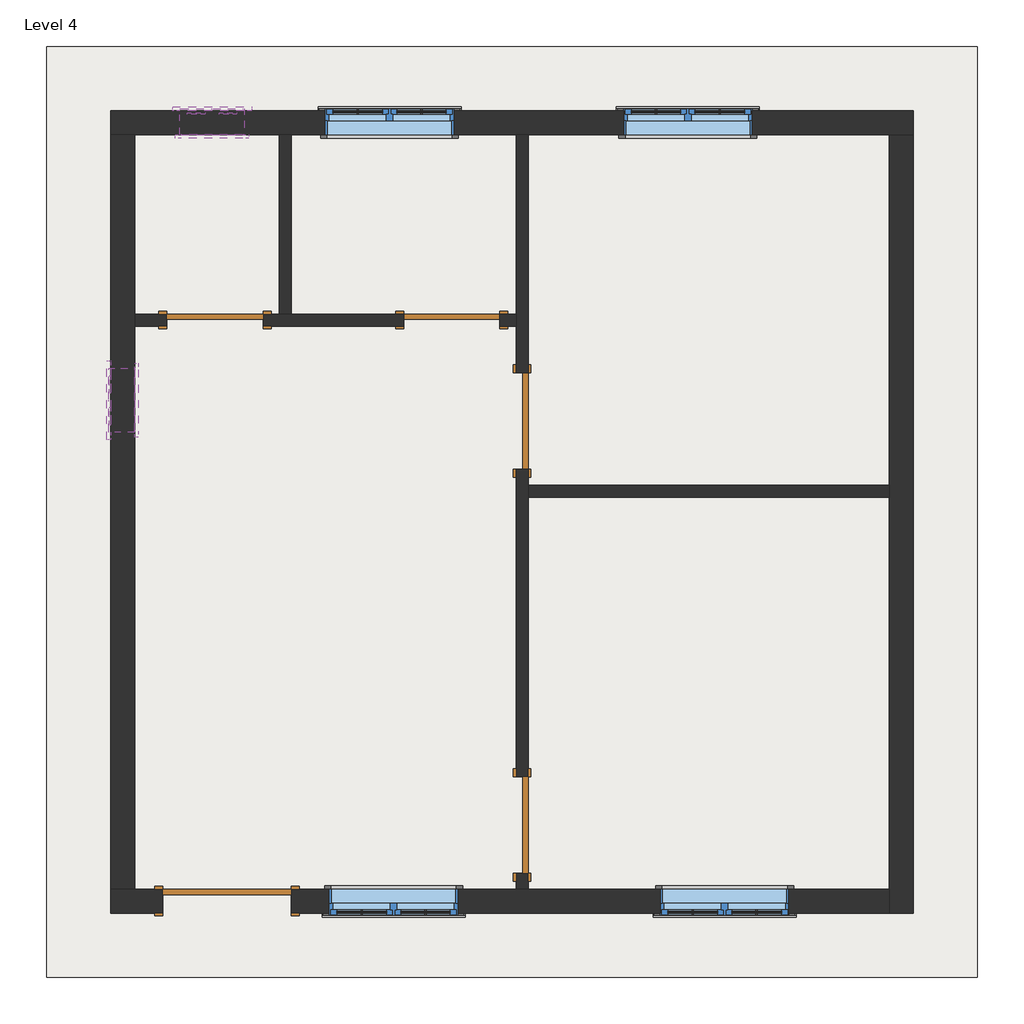
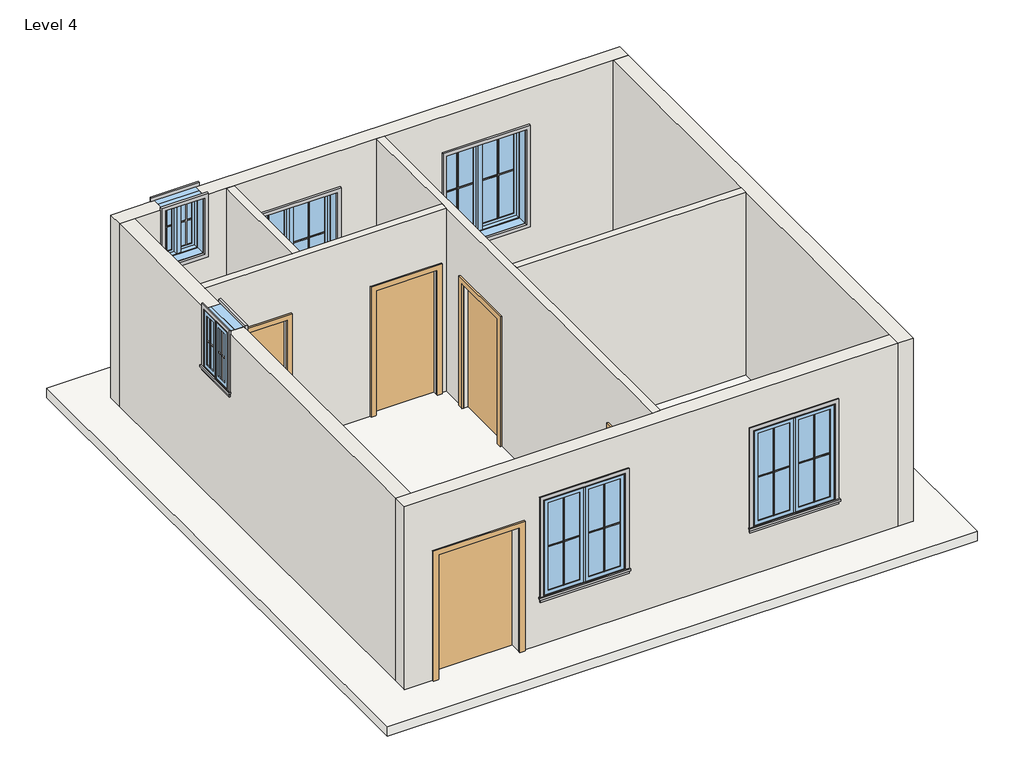
# One storey, incomplete: 24 proxies, 8 walls, 6 windows, 5 doors, 1 roof.
"""IFC4 building model written with IfcOpenShell, lengths in millimetres."""

from ifc_helpers import new_model, si_unit, frame, origin, place, context, project, spatial, polyline, outline, extrude, faceted_brep, transform, mapped, element, save
from components import muntin_pattern_2x2_muntin_pattern_2x2_6dad3731, muntin_pattern_2x2_muntin_pattern_2x2_a30a3345, muntin_pattern_2x2_muntin_pattern_2x2_53152e2c, muntin_pattern_2x2_muntin_pattern_2x2_e8f3e573, trim_window_exterior_flat_with_sill_92b9b949, trim_window_exterior_flat_with_sill_a665a915, trim_window_interior_flat_picture_frame_3bb882cf, trim_window_interior_flat_picture_frame_d485c387, door_e5f9f3c4, door_f4c4cdf2, window_c417fced, window_8377141f

model = new_model("IFC4")

# Units and contexts
model_context = context("Model", 3, world=origin())
ifc_project = project(units=[si_unit("LENGTHUNIT", "METRE", prefix="MILLI")], contexts=[model_context])

# Site, building, storey
site = spatial("IfcSite", under=ifc_project)
building = spatial("IfcBuilding", under=site)
storey = spatial("IfcBuildingStorey", under=building, Name="Level 4", Elevation=9144.0)

# Proxies
placement = place(None, origin())
muntin_pattern_2x2_muntin_pattern_2x2_shape = muntin_pattern_2x2_muntin_pattern_2x2_6dad3731(model_context)
element("IfcBuildingElementProxy", 1, Name="Muntin Pattern_2x2 : Muntin Pattern_2x2", ObjectType="Muntin Pattern_2x2 : Muntin Pattern_2x2", at=placement, inside=storey, context=model_context, shape_type="MappedRepresentation", body=[
    mapped(muntin_pattern_2x2_muntin_pattern_2x2_shape, transform((6192.8375, 13960.475, 10128.25), x_axis=(1.0, 0.0, 0.0), y_axis=(0.0, 1.0, 0.0), z_axis=(0.0, 0.0, 1.0))),
])
element("IfcBuildingElementProxy", 2, Name="Muntin Pattern_2x2 : Muntin Pattern_2x2", ObjectType="Muntin Pattern_2x2 : Muntin Pattern_2x2", at=placement, inside=storey, context=model_context, shape_type="MappedRepresentation", body=[
    mapped(muntin_pattern_2x2_muntin_pattern_2x2_shape, transform((7148.5125, 6359.525, 10128.25), x_axis=(-1.0, 0.0, 0.0), y_axis=(0.0, -1.0, 0.0), z_axis=(0.0, 0.0, 1.0))),
])
element("IfcBuildingElementProxy", 3, Name="Muntin Pattern_2x2 : Muntin Pattern_2x2", ObjectType="Muntin Pattern_2x2 : Muntin Pattern_2x2", at=placement, inside=storey, context=model_context, shape_type="MappedRepresentation", body=[
    mapped(muntin_pattern_2x2_muntin_pattern_2x2_shape, transform((4005.2625, 6359.525, 10128.25), x_axis=(-1.0, 0.0, 0.0), y_axis=(0.0, -1.0, 0.0), z_axis=(0.0, 0.0, 1.0))),
])
element("IfcBuildingElementProxy", 4, Name="Muntin Pattern_2x2 : Muntin Pattern_2x2", ObjectType="Muntin Pattern_2x2 : Muntin Pattern_2x2", at=placement, inside=storey, context=model_context, shape_type="MappedRepresentation", body=[
    mapped(muntin_pattern_2x2_muntin_pattern_2x2_shape, transform((3360.7375, 13960.475, 10128.25), x_axis=(1.0, 0.0, 0.0), y_axis=(0.0, 1.0, 0.0), z_axis=(0.0, 0.0, 1.0))),
])
muntin_pattern_2x2_muntin_pattern_2x2_2_shape = muntin_pattern_2x2_muntin_pattern_2x2_a30a3345(model_context)
element("IfcBuildingElementProxy", 5, Name="Muntin Pattern_2x2 : Muntin Pattern_2x2", ObjectType="Muntin Pattern_2x2 : Muntin Pattern_2x2", at=placement, inside=storey, context=model_context, shape_type="MappedRepresentation", body=[
    mapped(muntin_pattern_2x2_muntin_pattern_2x2_2_shape, transform((6799.2625, 13960.475, 10128.25), x_axis=(-1.0, 0.0, 0.0), y_axis=(0.0, -1.0, 0.0), z_axis=(0.0, 0.0, 1.0))),
])
element("IfcBuildingElementProxy", 6, Name="Muntin Pattern_2x2 : Muntin Pattern_2x2", ObjectType="Muntin Pattern_2x2 : Muntin Pattern_2x2", at=placement, inside=storey, context=model_context, shape_type="MappedRepresentation", body=[
    mapped(muntin_pattern_2x2_muntin_pattern_2x2_2_shape, transform((6542.0875, 6359.525, 10128.25), x_axis=(1.0, 0.0, 0.0), y_axis=(0.0, 1.0, 0.0), z_axis=(0.0, 0.0, 1.0))),
])
element("IfcBuildingElementProxy", 7, Name="Muntin Pattern_2x2 : Muntin Pattern_2x2", ObjectType="Muntin Pattern_2x2 : Muntin Pattern_2x2", at=placement, inside=storey, context=model_context, shape_type="MappedRepresentation", body=[
    mapped(muntin_pattern_2x2_muntin_pattern_2x2_2_shape, transform((3398.8375, 6359.525, 10128.25), x_axis=(1.0, 0.0, 0.0), y_axis=(0.0, 1.0, 0.0), z_axis=(0.0, 0.0, 1.0))),
])
element("IfcBuildingElementProxy", 8, Name="Muntin Pattern_2x2 : Muntin Pattern_2x2", ObjectType="Muntin Pattern_2x2 : Muntin Pattern_2x2", at=placement, inside=storey, context=model_context, shape_type="MappedRepresentation", body=[
    mapped(muntin_pattern_2x2_muntin_pattern_2x2_2_shape, transform((3967.1625, 13960.475, 10128.25), x_axis=(-1.0, 0.0, 0.0), y_axis=(0.0, -1.0, 0.0), z_axis=(0.0, 0.0, 1.0))),
])
muntin_pattern_2x2_muntin_pattern_2x2_3_shape = muntin_pattern_2x2_muntin_pattern_2x2_53152e2c(model_context)
element("IfcBuildingElementProxy", 9, Name="Muntin Pattern_2x2 : Muntin Pattern_2x2", ObjectType="Muntin Pattern_2x2 : Muntin Pattern_2x2", at=placement, inside=storey, context=model_context, shape_type="MappedRepresentation", body=[
    mapped(muntin_pattern_2x2_muntin_pattern_2x2_3_shape, transform((1025.525, 11069.6375, 11347.45), x_axis=(0.0, 1.0, 0.0), y_axis=(-1.0, 0.0, 0.0), z_axis=(0.0, 0.0, 1.0))),
])
element("IfcBuildingElementProxy", 10, Name="Muntin Pattern_2x2 : Muntin Pattern_2x2", ObjectType="Muntin Pattern_2x2 : Muntin Pattern_2x2", at=placement, inside=storey, context=model_context, shape_type="MappedRepresentation", body=[
    mapped(muntin_pattern_2x2_muntin_pattern_2x2_3_shape, transform((1827.2125, 13960.475, 11347.45), x_axis=(1.0, 0.0, 0.0), y_axis=(0.0, 1.0, 0.0), z_axis=(0.0, 0.0, 1.0))),
])
muntin_pattern_2x2_muntin_pattern_2x2_4_shape = muntin_pattern_2x2_muntin_pattern_2x2_e8f3e573(model_context)
element("IfcBuildingElementProxy", 11, Name="Muntin Pattern_2x2 : Muntin Pattern_2x2", ObjectType="Muntin Pattern_2x2 : Muntin Pattern_2x2", at=placement, inside=storey, context=model_context, shape_type="MappedRepresentation", body=[
    mapped(muntin_pattern_2x2_muntin_pattern_2x2_4_shape, transform((1025.525, 11371.2625, 11347.45), x_axis=(0.0, -1.0, 0.0), y_axis=(1.0, 0.0, 0.0), z_axis=(0.0, 0.0, 1.0))),
])
element("IfcBuildingElementProxy", 12, Name="Muntin Pattern_2x2 : Muntin Pattern_2x2", ObjectType="Muntin Pattern_2x2 : Muntin Pattern_2x2", at=placement, inside=storey, context=model_context, shape_type="MappedRepresentation", body=[
    mapped(muntin_pattern_2x2_muntin_pattern_2x2_4_shape, transform((2128.8375, 13960.475, 11347.45), x_axis=(-1.0, 0.0, 0.0), y_axis=(0.0, -1.0, 0.0), z_axis=(0.0, 0.0, 1.0))),
])
trim_window_exterior_flat_with_sill_shape = trim_window_exterior_flat_with_sill_92b9b949(model_context)
element("IfcBuildingElementProxy", 13, Name="Trim-Window-Exterior-Flat : with Sill", ObjectType="Trim-Window-Exterior-Flat : with Sill", at=placement, inside=storey, context=model_context, shape_type="MappedRepresentation", body=[
    mapped(trim_window_exterior_flat_with_sill_shape, transform((6496.05, 13970.0, 11582.4), x_axis=(-1.0, 0.0, 0.0), y_axis=(0.0, 0.0, 1.0), z_axis=(0.0, 1.0, 0.0))),
])
element("IfcBuildingElementProxy", 14, Name="Trim-Window-Exterior-Flat : with Sill", ObjectType="Trim-Window-Exterior-Flat : with Sill", at=placement, inside=storey, context=model_context, shape_type="MappedRepresentation", body=[
    mapped(trim_window_exterior_flat_with_sill_shape, transform((6845.3, 6350.0, 11582.4), x_axis=(1.0, 0.0, 0.0), y_axis=(0.0, 0.0, 1.0), z_axis=(0.0, -1.0, 0.0))),
])
element("IfcBuildingElementProxy", 15, Name="Trim-Window-Exterior-Flat : with Sill", ObjectType="Trim-Window-Exterior-Flat : with Sill", at=placement, inside=storey, context=model_context, shape_type="MappedRepresentation", body=[
    mapped(trim_window_exterior_flat_with_sill_shape, transform((3702.05, 6350.0, 11582.4), x_axis=(1.0, 0.0, 0.0), y_axis=(0.0, 0.0, 1.0), z_axis=(0.0, -1.0, 0.0))),
])
element("IfcBuildingElementProxy", 16, Name="Trim-Window-Exterior-Flat : with Sill", ObjectType="Trim-Window-Exterior-Flat : with Sill", at=placement, inside=storey, context=model_context, shape_type="MappedRepresentation", body=[
    mapped(trim_window_exterior_flat_with_sill_shape, transform((3663.95, 13970.0, 11582.4), x_axis=(-1.0, 0.0, 0.0), y_axis=(0.0, 0.0, 1.0), z_axis=(0.0, 1.0, 0.0))),
])
trim_window_exterior_flat_with_sill_2_shape = trim_window_exterior_flat_with_sill_a665a915(model_context)
element("IfcBuildingElementProxy", 17, Name="Trim-Window-Exterior-Flat : with Sill", ObjectType="Trim-Window-Exterior-Flat : with Sill", at=placement, inside=storey, context=model_context, shape_type="MappedRepresentation", body=[
    mapped(trim_window_exterior_flat_with_sill_2_shape, transform((1016.0, 11220.45, 12192.0), x_axis=(0.0, -1.0, 0.0), y_axis=(0.0, 0.0, 1.0), z_axis=(-1.0, 0.0, 0.0))),
])
element("IfcBuildingElementProxy", 18, Name="Trim-Window-Exterior-Flat : with Sill", ObjectType="Trim-Window-Exterior-Flat : with Sill", at=placement, inside=storey, context=model_context, shape_type="MappedRepresentation", body=[
    mapped(trim_window_exterior_flat_with_sill_2_shape, transform((1978.025, 13970.0, 12192.0), x_axis=(-1.0, 0.0, 0.0), y_axis=(0.0, 0.0, 1.0), z_axis=(0.0, 1.0, 0.0))),
])
trim_window_interior_flat_picture_frame_shape = trim_window_interior_flat_picture_frame_3bb882cf(model_context)
element("IfcBuildingElementProxy", 19, Name="Trim-Window-Interior-Flat : Picture Frame", ObjectType="Trim-Window-Interior-Flat : Picture Frame", at=placement, inside=storey, context=model_context, shape_type="MappedRepresentation", body=[
    mapped(trim_window_interior_flat_picture_frame_shape, transform((6496.05, 13741.4, 11582.4), x_axis=(1.0, 0.0, 0.0), y_axis=(0.0, 0.0, 1.0), z_axis=(0.0, -1.0, 0.0))),
])
element("IfcBuildingElementProxy", 20, Name="Trim-Window-Interior-Flat : Picture Frame", ObjectType="Trim-Window-Interior-Flat : Picture Frame", at=placement, inside=storey, context=model_context, shape_type="MappedRepresentation", body=[
    mapped(trim_window_interior_flat_picture_frame_shape, transform((6845.3, 6578.6, 11582.4), x_axis=(-1.0, 0.0, 0.0), y_axis=(0.0, 0.0, 1.0), z_axis=(0.0, 1.0, 0.0))),
])
element("IfcBuildingElementProxy", 21, Name="Trim-Window-Interior-Flat : Picture Frame", ObjectType="Trim-Window-Interior-Flat : Picture Frame", at=placement, inside=storey, context=model_context, shape_type="MappedRepresentation", body=[
    mapped(trim_window_interior_flat_picture_frame_shape, transform((3702.05, 6578.6, 11582.4), x_axis=(-1.0, 0.0, 0.0), y_axis=(0.0, 0.0, 1.0), z_axis=(0.0, 1.0, 0.0))),
])
element("IfcBuildingElementProxy", 22, Name="Trim-Window-Interior-Flat : Picture Frame", ObjectType="Trim-Window-Interior-Flat : Picture Frame", at=placement, inside=storey, context=model_context, shape_type="MappedRepresentation", body=[
    mapped(trim_window_interior_flat_picture_frame_shape, transform((3663.95, 13741.4, 11582.4), x_axis=(1.0, 0.0, 0.0), y_axis=(0.0, 0.0, 1.0), z_axis=(0.0, -1.0, 0.0))),
])
trim_window_interior_flat_picture_frame_2_shape = trim_window_interior_flat_picture_frame_d485c387(model_context)
element("IfcBuildingElementProxy", 23, Name="Trim-Window-Interior-Flat : Picture Frame", ObjectType="Trim-Window-Interior-Flat : Picture Frame", at=placement, inside=storey, context=model_context, shape_type="MappedRepresentation", body=[
    mapped(trim_window_interior_flat_picture_frame_2_shape, transform((1244.6, 11220.45, 12192.0), x_axis=(0.0, 1.0, 0.0), y_axis=(0.0, 0.0, 1.0), z_axis=(1.0, 0.0, 0.0))),
])
element("IfcBuildingElementProxy", 24, Name="Trim-Window-Interior-Flat : Picture Frame", ObjectType="Trim-Window-Interior-Flat : Picture Frame", at=placement, inside=storey, context=model_context, shape_type="MappedRepresentation", body=[
    mapped(trim_window_interior_flat_picture_frame_2_shape, transform((1978.025, 13741.4, 12192.0), x_axis=(1.0, 0.0, 0.0), y_axis=(0.0, 0.0, 1.0), z_axis=(0.0, -1.0, 0.0))),
])

# Doors
door_shape = door_e5f9f3c4(model_context)
element("IfcDoor", 25, ObjectType="Single-Flush : 36\" x 84\"", at=placement, inside=storey, context=model_context, shape_type="MappedRepresentation", body=[
    mapped(door_shape, transform((2006.6, 11982.45, 9144.0), x_axis=(1.0, 0.0, 0.0), y_axis=(0.0, 1.0, 0.0), z_axis=(0.0, 0.0, 1.0))),
])
element("IfcDoor", 26, ObjectType="Single-Flush : 36\" x 84\"", at=placement, inside=storey, context=model_context, shape_type="MappedRepresentation", body=[
    mapped(door_shape, transform((4254.5, 11982.45, 9144.0), x_axis=(1.0, 0.0, 0.0), y_axis=(0.0, 1.0, 0.0), z_axis=(0.0, 0.0, 1.0))),
])
element("IfcDoor", 27, ObjectType="Single-Flush : 36\" x 84\"", at=placement, inside=storey, context=model_context, shape_type="MappedRepresentation", body=[
    mapped(door_shape, transform((4921.25, 11023.6, 9144.0), x_axis=(0.0, -1.0, 0.0), y_axis=(1.0, 0.0, 0.0), z_axis=(0.0, 0.0, 1.0))),
])
element("IfcDoor", 28, ObjectType="Single-Flush : 36\" x 84\"", at=placement, inside=storey, context=model_context, shape_type="MappedRepresentation", body=[
    mapped(door_shape, transform((4921.25, 7188.2, 9144.0), x_axis=(0.0, -1.0, 0.0), y_axis=(1.0, 0.0, 0.0), z_axis=(0.0, 0.0, 1.0))),
])
door_2_shape = door_f4c4cdf2(model_context)
element("IfcDoor", 29, ObjectType="Single-Flush : 48\" x 84\"", at=placement, inside=storey, context=model_context, shape_type="MappedRepresentation", body=[
    mapped(door_2_shape, transform((2120.9, 6464.3, 9144.0), x_axis=(-1.0, 0.0, 0.0), y_axis=(0.0, -1.0, 0.0), z_axis=(0.0, 0.0, 1.0))),
])

# Roof
element("IfcRoof", 30, ObjectType="Generic - 12\"", at=placement, inside=storey, context=model_context, shape_type="SweptSolid", body=[
    extrude(outline(polyline([(406.4, 14579.6), (9245.6, 14579.6), (9245.6, 5740.4), (406.4, 5740.4), (406.4, 14579.6)])), frame((0.0, 0.0, 9144.0), z_axis=(0.0, 0.0, 1.0), x_axis=(1.0, 0.0, 0.0)), (0.0, 0.0, 1.0), 152.4),
])

# Walls
element("IfcWall", 31, ObjectType="Generic - 5\"", at=placement, inside=storey, context=model_context, shape_type="SweptSolid", body=[
    extrude(outline(polyline([(2616.2, 12039.6), (2616.2, 13741.4), (2730.5, 13741.4), (2730.5, 12039.6), (2616.2, 12039.6)])), frame((0.0, 0.0, 9144.0), z_axis=(0.0, 0.0, 1.0), x_axis=(1.0, 0.0, 0.0)), (0.0, 0.0, 1.0), 3048.0),
])
element("IfcWall", 32, ObjectType="Generic - 5\"", at=placement, inside=storey, context=model_context, shape_type="Brep", body=[
    faceted_brep([(4711.7, 11925.3, 11277.6), (4711.7, 11925.3, 9144.0), (4864.1, 11925.3, 9144.0), (4864.1, 11925.3, 12192.0), (1244.6, 11925.3, 12192.0), (1244.6, 11925.3, 9144.0), (1549.4, 11925.3, 9144.0), (1549.4, 11925.3, 11277.6), (2463.8, 11925.3, 11277.6), (2463.8, 11925.3, 9144.0), (3797.3, 11925.3, 9144.0), (3797.3, 11925.3, 11277.6), (4864.1, 12039.6, 9144.0), (4711.7, 12039.6, 9144.0), (4711.7, 12039.6, 11277.6), (3797.3, 12039.6, 11277.6), (3797.3, 12039.6, 9144.0), (2730.5, 12039.6, 9144.0), (2616.2, 12039.6, 9144.0), (2463.8, 12039.6, 9144.0), (2463.8, 12039.6, 11277.6), (1549.4, 12039.6, 11277.6), (1549.4, 12039.6, 9144.0), (1244.6, 12039.6, 9144.0), (1244.6, 12039.6, 12192.0), (2616.2, 12039.6, 12192.0), (2730.5, 12039.6, 12192.0), (4864.1, 12039.6, 12192.0)], [[[0, 1, 2, 3, 4, 5, 6, 7, 8, 9, 10, 11]], [[12, 13, 14, 15, 16, 17, 18, 19, 20, 21, 22, 23, 24, 25, 26, 27]], [[6, 5, 23, 22]], [[10, 9, 19, 18, 17, 16]], [[2, 1, 13, 12]], [[4, 3, 27, 26, 25, 24]], [[5, 4, 24, 23]], [[3, 2, 12, 27]], [[20, 19, 9, 8]], [[21, 20, 8, 7]], [[22, 21, 7, 6]], [[14, 13, 1, 0]], [[15, 14, 0, 11]], [[16, 15, 11, 10]]]),
])
element("IfcWall", 33, ObjectType="Generic - 5\"", at=placement, inside=storey, context=model_context, shape_type="Brep", body=[
    faceted_brep([(4864.1, 6731.0, 11277.6), (4864.1, 6731.0, 9144.0), (4864.1, 6578.6, 9144.0), (4864.1, 6578.6, 12192.0), (4864.1, 11925.3, 12192.0), (4864.1, 12039.6, 12192.0), (4864.1, 13741.4, 12192.0), (4864.1, 13741.4, 9144.0), (4864.1, 12039.6, 9144.0), (4864.1, 11925.3, 9144.0), (4864.1, 11480.8, 9144.0), (4864.1, 11480.8, 11277.6), (4864.1, 10566.4, 11277.6), (4864.1, 10566.4, 9144.0), (4864.1, 7645.4, 9144.0), (4864.1, 7645.4, 11277.6), (4978.4, 6578.6, 9144.0), (4978.4, 6731.0, 9144.0), (4978.4, 6731.0, 11277.6), (4978.4, 7645.4, 11277.6), (4978.4, 7645.4, 9144.0), (4978.4, 10299.7, 9144.0), (4978.4, 10414.0, 9144.0), (4978.4, 10566.4, 9144.0), (4978.4, 10566.4, 11277.6), (4978.4, 11480.8, 11277.6), (4978.4, 11480.8, 9144.0), (4978.4, 13741.4, 9144.0), (4978.4, 13741.4, 12192.0), (4978.4, 10414.0, 12192.0), (4978.4, 10299.7, 12192.0), (4978.4, 6578.6, 12192.0)], [[[0, 1, 2, 3, 4, 5, 6, 7, 8, 9, 10, 11, 12, 13, 14, 15]], [[16, 17, 18, 19, 20, 21, 22, 23, 24, 25, 26, 27, 28, 29, 30, 31]], [[10, 9, 8, 7, 27, 26]], [[14, 13, 23, 22, 21, 20]], [[2, 1, 17, 16]], [[6, 5, 4, 3, 31, 30, 29, 28]], [[7, 6, 28, 27]], [[3, 2, 16, 31]], [[24, 23, 13, 12]], [[25, 24, 12, 11]], [[26, 25, 11, 10]], [[18, 17, 1, 0]], [[19, 18, 0, 15]], [[20, 19, 15, 14]]]),
])
element("IfcWall", 34, ObjectType="Generic - 5\"", at=placement, inside=storey, context=model_context, shape_type="SweptSolid", body=[
    extrude(outline(polyline([(8407.4, 10299.7), (4978.4, 10299.7), (4978.4, 10414.0), (8407.4, 10414.0), (8407.4, 10299.7)])), frame((0.0, 0.0, 9144.0), z_axis=(0.0, 0.0, 1.0), x_axis=(1.0, 0.0, 0.0)), (0.0, 0.0, 1.0), 3048.0),
])
element("IfcWall", 35, ObjectType="Generic - 8\"", at=placement, inside=storey, context=model_context, shape_type="Brep", body=[
    faceted_brep([(1016.0, 13741.4, 9144.0), (1244.6, 13741.4, 9144.0), (2616.2, 13741.4, 9144.0), (2730.5, 13741.4, 9144.0), (4864.1, 13741.4, 9144.0), (4978.4, 13741.4, 9144.0), (8407.4, 13741.4, 9144.0), (8636.0, 13741.4, 9144.0), (8636.0, 13741.4, 12192.0), (8407.4, 13741.4, 12192.0), (4978.4, 13741.4, 12192.0), (4864.1, 13741.4, 12192.0), (2730.5, 13741.4, 12192.0), (2616.2, 13741.4, 12192.0), (2282.825, 13741.4, 12192.0), (2282.825, 13741.4, 11277.6), (1673.225, 13741.4, 11277.6), (1673.225, 13741.4, 12192.0), (1244.6, 13741.4, 12192.0), (1016.0, 13741.4, 12192.0), (7105.65, 13741.4, 11582.4), (7105.65, 13741.4, 10058.4), (5886.45, 13741.4, 10058.4), (5886.45, 13741.4, 11582.4), (4273.55, 13741.4, 11582.4), (4273.55, 13741.4, 10058.4), (3054.35, 13741.4, 10058.4), (3054.35, 13741.4, 11582.4), (8636.0, 13970.0, 9144.0), (1016.0, 13970.0, 9144.0), (1016.0, 13970.0, 12192.0), (1673.225, 13970.0, 12192.0), (1673.225, 13970.0, 11277.6), (2282.825, 13970.0, 11277.6), (2282.825, 13970.0, 12192.0), (8636.0, 13970.0, 12192.0), (7105.65, 13970.0, 10058.4), (7105.65, 13970.0, 11582.4), (5886.45, 13970.0, 11582.4), (5886.45, 13970.0, 10058.4), (4273.55, 13970.0, 10058.4), (4273.55, 13970.0, 11582.4), (3054.35, 13970.0, 11582.4), (3054.35, 13970.0, 10058.4)], [[[0, 1, 2, 3, 4, 5, 6, 7, 8, 9, 10, 11, 12, 13, 14, 15, 16, 17, 18, 19], [20, 21, 22, 23], [24, 25, 26, 27]], [[28, 29, 30, 31, 32, 33, 34, 35], [36, 37, 38, 39], [40, 41, 42, 43]], [[7, 6, 5, 4, 3, 2, 1, 0, 29, 28]], [[8, 35, 34, 14, 13, 12, 11, 10, 9]], [[30, 19, 18, 17, 31]], [[8, 7, 28, 35]], [[0, 19, 30, 29]], [[21, 20, 37, 36]], [[22, 21, 36, 39]], [[23, 22, 39, 38]], [[20, 23, 38, 37]], [[25, 24, 41, 40]], [[26, 25, 40, 43]], [[27, 26, 43, 42]], [[24, 27, 42, 41]], [[33, 15, 14, 34]], [[15, 33, 32, 16]], [[16, 32, 31, 17]]]),
])
element("IfcWall", 36, ObjectType="Generic - 8\"", at=placement, inside=storey, context=model_context, shape_type="Brep", body=[
    faceted_brep([(8407.4, 13741.4, 9144.0), (8407.4, 10414.0, 9144.0), (8407.4, 10299.7, 9144.0), (8407.4, 6578.6, 9144.0), (8407.4, 6350.0, 9144.0), (8407.4, 6350.0, 12192.0), (8407.4, 6578.6, 12192.0), (8407.4, 10299.7, 12192.0), (8407.4, 10414.0, 12192.0), (8407.4, 13741.4, 12192.0), (8636.0, 13741.4, 9144.0), (8636.0, 13741.4, 12192.0), (8636.0, 6350.0, 12192.0), (8636.0, 6350.0, 9144.0)], [[[0, 1, 2, 3, 4, 5, 6, 7, 8, 9]], [[10, 11, 12, 13]], [[4, 3, 2, 1, 0, 10, 13]], [[9, 8, 7, 6, 5, 12, 11]], [[0, 9, 11, 10]], [[5, 4, 13, 12]]]),
])
element("IfcWall", 37, ObjectType="Generic - 8\"", at=placement, inside=storey, context=model_context, shape_type="Brep", body=[
    faceted_brep([(1511.3, 6578.6, 11277.6), (1511.3, 6578.6, 9144.0), (1244.6, 6578.6, 9144.0), (1016.0, 6578.6, 9144.0), (1016.0, 6578.6, 12192.0), (1244.6, 6578.6, 12192.0), (4864.1, 6578.6, 12192.0), (4978.4, 6578.6, 12192.0), (8407.4, 6578.6, 12192.0), (8407.4, 6578.6, 9144.0), (4978.4, 6578.6, 9144.0), (4864.1, 6578.6, 9144.0), (2730.5, 6578.6, 9144.0), (2730.5, 6578.6, 11277.6), (6235.7, 6578.6, 11582.4), (6235.7, 6578.6, 10058.4), (7454.9, 6578.6, 10058.4), (7454.9, 6578.6, 11582.4), (3092.45, 6578.6, 11582.4), (3092.45, 6578.6, 10058.4), (4311.65, 6578.6, 10058.4), (4311.65, 6578.6, 11582.4), (1016.0, 6350.0, 9144.0), (1511.3, 6350.0, 9144.0), (1511.3, 6350.0, 11277.6), (2730.5, 6350.0, 11277.6), (2730.5, 6350.0, 9144.0), (8407.4, 6350.0, 9144.0), (8407.4, 6350.0, 12192.0), (1016.0, 6350.0, 12192.0), (6235.7, 6350.0, 11582.4), (7454.9, 6350.0, 11582.4), (7454.9, 6350.0, 10058.4), (6235.7, 6350.0, 10058.4), (3092.45, 6350.0, 11582.4), (4311.65, 6350.0, 11582.4), (4311.65, 6350.0, 10058.4), (3092.45, 6350.0, 10058.4)], [[[0, 1, 2, 3, 4, 5, 6, 7, 8, 9, 10, 11, 12, 13], [14, 15, 16, 17], [18, 19, 20, 21]], [[22, 23, 24, 25, 26, 27, 28, 29], [30, 31, 32, 33], [34, 35, 36, 37]], [[3, 2, 1, 23, 22]], [[12, 11, 10, 9, 27, 26]], [[8, 7, 6, 5, 4, 29, 28]], [[9, 8, 28, 27]], [[4, 3, 22, 29]], [[24, 23, 1, 0]], [[25, 24, 0, 13]], [[26, 25, 13, 12]], [[15, 14, 30, 33]], [[16, 15, 33, 32]], [[17, 16, 32, 31]], [[14, 17, 31, 30]], [[19, 18, 34, 37]], [[20, 19, 37, 36]], [[21, 20, 36, 35]], [[18, 21, 35, 34]]]),
])
element("IfcWall", 38, ObjectType="Generic - 8\"", at=placement, inside=storey, context=model_context, shape_type="Brep", body=[
    faceted_brep([(1244.6, 6578.6, 9144.0), (1244.6, 11925.3, 9144.0), (1244.6, 12039.6, 9144.0), (1244.6, 13741.4, 9144.0), (1244.6, 13741.4, 12192.0), (1244.6, 12039.6, 12192.0), (1244.6, 11925.3, 12192.0), (1244.6, 11525.25, 12192.0), (1244.6, 11525.25, 11277.6), (1244.6, 10915.65, 11277.6), (1244.6, 10915.65, 12192.0), (1244.6, 6578.6, 12192.0), (1016.0, 13741.4, 9144.0), (1016.0, 6578.6, 9144.0), (1016.0, 6578.6, 12192.0), (1016.0, 10915.65, 12192.0), (1016.0, 10915.65, 11277.6), (1016.0, 11525.25, 11277.6), (1016.0, 11525.25, 12192.0), (1016.0, 13741.4, 12192.0)], [[[0, 1, 2, 3, 4, 5, 6, 7, 8, 9, 10, 11]], [[12, 13, 14, 15, 16, 17, 18, 19]], [[3, 2, 1, 0, 13, 12]], [[14, 11, 10, 15]], [[4, 19, 18, 7, 6, 5]], [[4, 3, 12, 19]], [[0, 11, 14, 13]], [[17, 8, 7, 18]], [[8, 17, 16, 9]], [[9, 16, 15, 10]]]),
])

# Windows
window_shape = window_c417fced(model_context)
element("IfcWindow", 39, ObjectType="Window-Casement-Double : 24\" x 36\"", at=placement, inside=storey, context=model_context, shape_type="MappedRepresentation", body=[
    mapped(window_shape, transform((1130.3, 11220.45, 10363.2), x_axis=(0.0, 1.0, 0.0), y_axis=(-1.0, 0.0, 0.0), z_axis=(0.0, 0.0, 1.0))),
])
element("IfcWindow", 40, ObjectType="Window-Casement-Double : 24\" x 36\"", at=placement, inside=storey, context=model_context, shape_type="MappedRepresentation", body=[
    mapped(window_shape, transform((1978.025, 13855.7, 10363.2), x_axis=(1.0, 0.0, 0.0), y_axis=(0.0, 1.0, 0.0), z_axis=(0.0, 0.0, 1.0))),
])
window_2_shape = window_8377141f(model_context)
element("IfcWindow", 41, ObjectType="Window-Casement-Double : 48\" x 60\"", at=placement, inside=storey, context=model_context, shape_type="MappedRepresentation", body=[
    mapped(window_2_shape, transform((6496.05, 13855.7, 9144.0), x_axis=(1.0, 0.0, 0.0), y_axis=(0.0, 1.0, 0.0), z_axis=(0.0, 0.0, 1.0))),
])
element("IfcWindow", 42, ObjectType="Window-Casement-Double : 48\" x 60\"", at=placement, inside=storey, context=model_context, shape_type="MappedRepresentation", body=[
    mapped(window_2_shape, transform((6845.3, 6464.3, 9144.0), x_axis=(-1.0, 0.0, 0.0), y_axis=(0.0, -1.0, 0.0), z_axis=(0.0, 0.0, 1.0))),
])
element("IfcWindow", 43, ObjectType="Window-Casement-Double : 48\" x 60\"", at=placement, inside=storey, context=model_context, shape_type="MappedRepresentation", body=[
    mapped(window_2_shape, transform((3702.05, 6464.3, 9144.0), x_axis=(-1.0, 0.0, 0.0), y_axis=(0.0, -1.0, 0.0), z_axis=(0.0, 0.0, 1.0))),
])
element("IfcWindow", 44, ObjectType="Window-Casement-Double : 48\" x 60\"", at=placement, inside=storey, context=model_context, shape_type="MappedRepresentation", body=[
    mapped(window_2_shape, transform((3663.95, 13855.7, 9144.0), x_axis=(1.0, 0.0, 0.0), y_axis=(0.0, 1.0, 0.0), z_axis=(0.0, 0.0, 1.0))),
])

save(model, "model.ifc")

# Revit data of these elements
# Type "Muntin Pattern_2x2 : Muntin Pattern_2x2"
#   Width [instance default] = 4' - 0"
#   Thickness = 0' - 0 1/2"
#   Height [instance default] = 4' - 0"
#   Distance = 0' - 0 3/4"
#   Interior Material [instance default] = none
#   Exterior Material [instance default] = none
#   Default Elevation = 0
# Type "Trim-Window-Exterior-Flat : with Sill"
#   Trim Width = 0' - 2 1/4"
#   Trim Thickness_Picture Frame = 0' - 1 1/4"
#   Trim Thickness_with Sill = 0' - 0 3/4"
#   Sill Thickness = 0' - 1 1/4"
#   Opening Width [instance default] = 2' - 0"
#   Opening Height [instance default] = 3' - 0"
#   Default Elevation = 4' - 0"
#   Sill = yes
#   Picture Frame = no
#   Trim Material [instance default] = none
# Type "Trim-Window-Interior-Flat : Picture Frame"
#   Trim Thickness_Picture Frame = 0' - 1 1/4"
#   Trim Width = 0' - 2 1/4"
#   Trim Thickness_with Sill = 0' - 0 3/4"
#   Sill Thickness = 0' - 1 1/4"
#   Opening Width [instance default] = 2' - 0"
#   Opening Height [instance default] = 3' - 0"
#   Default Elevation = 4' - 0"
#   Sill = no
#   Picture Frame = yes
#   Trim Material [instance default] = none
# Type "Single-Flush : 36\" x 84\""
#   Type Mark = "1"
#   Construction Type Id = "MDOOR"
#   Assembly Code = "C1020"
#   Analytic Construction = "Metal"
#   Thickness = 0' - 2"
#   Heat Transfer Coefficient (U) = 0.651978 BTU/(h·ft²·°F)
#   Height = 7' - 0"
#   Trim Projection Ext = 0' - 1"
#   Trim Projection Int = 0' - 1"
#   Trim Width = 0' - 3"
#   Width = 3' - 0"
#   Define Thermal Properties by = 1
#   Define Thermal Properties by = 1
#   Door Material = Door - Panel
#   Frame Material = Door - Frame
#   Visual Light Transmittance = 0
#   Solar Heat Gain Coefficient = 0
#   Function = (empty or 0)
#   Wall Closure = (empty or 0)
# Type "Single-Flush : 48\" x 84\""
#   Type Mark = "5"
#   Construction Type Id = "MDOOR"
#   Assembly Code = "C1020"
#   Analytic Construction = "Metal"
#   Thickness = 0' - 2"
#   Heat Transfer Coefficient (U) = 0.651978 BTU/(h·ft²·°F)
#   Height = 7' - 0"
#   Trim Projection Ext = 0' - 1"
#   Trim Projection Int = 0' - 1"
#   Trim Width = 0' - 3"
#   Width = 4' - 0"
#   Define Thermal Properties by = 1
#   Define Thermal Properties by = 1
#   Door Material = Door - Panel
#   Frame Material = Door - Frame
#   Visual Light Transmittance = 0
#   Solar Heat Gain Coefficient = 0
#   Function = (empty or 0)
#   Wall Closure = (empty or 0)
# Type "Generic - 12\""
#   Assembly Code = "B1020"
#   Layers, outside or top first: 0' - 6" no material (function 1)
# Type "Generic - 5\""
#   Assembly Code = "B2010"
#   Layers, outside or top first: 0' - 4 1/2" no material (function 1)
# Type "Generic - 8\""
#   Assembly Code = "B2010"
#   Layers, outside or top first: 0' - 9" "Parking Stripe" (function 1)
# Type "Window-Casement-Double : 24\" x 36\""
#   Type Mark = "14"
#   Fire Rating = "0.5h"
#   Assembly Code = "B2020100"
#   Analytic Construction = "Double glazing - domestic"
#   Frame Extension [instance default] = 0' - 0 1/4"
#   Window Inset [instance default] = 0' - 0"
#   Wall Thickness [instance default] = 0' - 6"
#   Interior Wall Closure [instance default] = 0' - 2 1/4"
#   Half Width = 1' - 0"
#   Visual Light Transmittance = 0.81
#   Thermal Resistance (R) = 1.8146 (h·ft²·°F)/BTU
#   Solar Heat Gain Coefficient = 0.76
#   Rough Width = 2' - 0 1/2"
#   Rough Height = 3' - 0 1/2"
#   Height = 3' - 0"
#   Heat Transfer Coefficient (U) = 0.5511 BTU/(h·ft²·°F)
#   Exterior Wall Closure [instance default] = 0' - 1 1/4"
#   Extension Jamb [instance default] = 0' - 2 1/4"
#   Default Sill Height = 3' - 0"
#   Width = 2' - 0"
#   Define Thermal Properties by = 0
#   Muntin Visibility = yes
#   Interior Trim Visibility [instance default] = yes
#   Exterior Trim Visibility [instance default] = yes
#   Extension Jamb Visibility [instance default] = yes
#   Interior Trim Material = Wood - Stained
#   Muntin Pattern = Muntin Pattern_2x2 : Muntin Pattern_2x2
#   Interior Trim = Trim-Window-Interior-Flat : Picture Frame
#   Interior Frame Material = Wood - Stained
#   Glass Panel Material = Glass
#   Exterior Trim Material = Clad - White
#   Exterior Trim = Trim-Window-Exterior-Flat : with Sill
#   Exterior Frame Material = Clad - White
#   Wall Closure = (empty or 0)
# Type "Window-Casement-Double : 48\" x 60\""
#   Type Mark = "17"
#   Fire Rating = "0.5h"
#   Assembly Code = "B2020100"
#   Analytic Construction = "Double glazing - domestic"
#   Frame Extension [instance default] = 0' - 0 1/4"
#   Window Inset [instance default] = 0' - 0"
#   Wall Thickness [instance default] = 0' - 6"
#   Interior Wall Closure [instance default] = 0' - 2 1/4"
#   Half Width = 2' - 0"
#   Visual Light Transmittance = 0.81
#   Thermal Resistance (R) = 1.8146 (h·ft²·°F)/BTU
#   Solar Heat Gain Coefficient = 0.76
#   Rough Width = 4' - 0 1/2"
#   Rough Height = 5' - 0 1/2"
#   Height = 5' - 0"
#   Heat Transfer Coefficient (U) = 0.5511 BTU/(h·ft²·°F)
#   Exterior Wall Closure [instance default] = 0' - 1 1/4"
#   Extension Jamb [instance default] = 0' - 2 1/4"
#   Default Sill Height = 3' - 0"
#   Width = 4' - 0"
#   Define Thermal Properties by = 0
#   Muntin Visibility = yes
#   Interior Trim Visibility [instance default] = yes
#   Exterior Trim Visibility [instance default] = yes
#   Extension Jamb Visibility [instance default] = yes
#   Interior Trim Material = Wood - Stained
#   Muntin Pattern = Muntin Pattern_2x2 : Muntin Pattern_2x2
#   Interior Trim = Trim-Window-Interior-Flat : Picture Frame
#   Interior Frame Material = Wood - Stained
#   Glass Panel Material = Glass
#   Exterior Trim Material = Clad - White
#   Exterior Trim = Trim-Window-Exterior-Flat : with Sill
#   Exterior Frame Material = Clad - White
#   Wall Closure = (empty or 0)
# Elements 1, 2, 3, 4, 5, 6, 7, 8 (IfcBuildingElementProxy, "Muntin Pattern_2x2 : Muntin Pattern_2x2")
#   Width = 1' - 6 5/8"
#   Height = 4' - 6 1/2"
#   Interior Material = Wood - Stained
#   Exterior Material = Clad - White
#   Phase Created = New Construction
#   Materials on its faces: "Clad - White", "Wood - Stained"
# Elements 9, 10, 11, 12 (IfcBuildingElementProxy, "Muntin Pattern_2x2 : Muntin Pattern_2x2")
#   Width = 0' - 6 5/8"
#   Height = 2' - 6 1/2"
#   Interior Material = Wood - Stained
#   Exterior Material = Clad - White
#   Phase Created = New Construction
#   Materials on its faces: "Clad - White", "Wood - Stained"
# Elements 13, 14, 15, 16 (IfcBuildingElementProxy, "Trim-Window-Exterior-Flat : with Sill")
#   Opening Width = 4' - 0"
#   Opening Height = 5' - 0"
#   Trim Material = Clad - White
#   Phase Created = New Construction
#   Materials on its faces: "Clad - White"
# Elements 17, 18 (IfcBuildingElementProxy, "Trim-Window-Exterior-Flat : with Sill")
#   Opening Width = 2' - 0"
#   Opening Height = 3' - 0"
#   Trim Material = Clad - White
#   Phase Created = New Construction
#   Materials on its faces: "Clad - White"
# Elements 19, 20, 21, 22 (IfcBuildingElementProxy, "Trim-Window-Interior-Flat : Picture Frame")
#   Opening Width = 4' - 0"
#   Opening Height = 5' - 0"
#   Trim Material = Wood - Stained
#   Phase Created = New Construction
#   Materials on its faces: "Wood - Stained"
# Elements 23, 24 (IfcBuildingElementProxy, "Trim-Window-Interior-Flat : Picture Frame")
#   Opening Width = 2' - 0"
#   Opening Height = 3' - 0"
#   Trim Material = Wood - Stained
#   Phase Created = New Construction
#   Materials on its faces: "Wood - Stained"
# Elements 25, 26, 27, 28 (IfcDoor, "Single-Flush : 36\" x 84\"")
#   Phase Created = New Construction
#   Materials on its faces: "Door - Frame", "Door - Panel"
# Element 29 (IfcDoor, "Single-Flush : 48\" x 84\"")
#   Phase Created = New Construction
#   Materials on its faces: "Door - Frame", "Door - Panel"
# Element 30 (IfcRoof, "Generic - 12\"")
#   built-in parameter 1001705 = 30.5 (stored number, unit not read)
#   built-in parameter 1001710 = 33615
#   Phase Created = New Construction
#   Materials on its faces: "Textile - Linen, Smooth", "Door - Panel"
# Elements 31, 32, 33, 34 (IfcWall, "Generic - 5\"")
#   Top Offset = 0' - 0"
#   Base Offset = 0' - 0"
#   wall height = 10' - 0"
#   Phase Created = New Construction
#   Base Constraint = Level 4
#   Top Constraint = Level 5
#   Materials on its faces: "Default Wall"
# Elements 35, 36, 37, 38 (IfcWall, "Generic - 8\"")
#   Top Offset = 0' - 0"
#   Base Offset = 0' - 0"
#   Unconnected Height = 10' - 0"
#   wall height = 10' - 0"
#   Phase Created = New Construction
#   Base Constraint = Level 4
#   Materials on its faces: "Parking Stripe", "Wood Planks"
# Element 39 (IfcWindow, "Window-Casement-Double : 24\" x 36\"")
#   Mark = "23"
#   Window Inset = 0' - 0"
#   Interior Wall Closure = 0' - 2 1/4"
#   Frame Extension = 0' - 0 1/4"
#   Exterior Wall Closure = 0' - 1 1/4"
#   Interior Trim Visibility = yes
#   Exterior Trim Visibility = yes
#   Phase Created = New Construction
#   Materials on its faces: "Wood - Stained", "Glass", "Clad - White"
# Element 40 (IfcWindow, "Window-Casement-Double : 24\" x 36\"")
#   Mark = "24"
#   Window Inset = 0' - 0"
#   Interior Wall Closure = 0' - 2 1/4"
#   Frame Extension = 0' - 0 1/4"
#   Exterior Wall Closure = 0' - 1 1/4"
#   Interior Trim Visibility = yes
#   Exterior Trim Visibility = yes
#   Phase Created = New Construction
#   Materials on its faces: "Wood - Stained", "Glass", "Clad - White"
# Element 41 (IfcWindow, "Window-Casement-Double : 48\" x 60\"")
#   Mark = "19"
#   Window Inset = 0' - 0"
#   Interior Wall Closure = 0' - 2 1/4"
#   Frame Extension = 0' - 0 1/4"
#   Exterior Wall Closure = 0' - 1 1/4"
#   Interior Trim Visibility = yes
#   Exterior Trim Visibility = yes
#   Phase Created = New Construction
#   Materials on its faces: "Wood - Stained", "Glass", "Clad - White"
# Element 42 (IfcWindow, "Window-Casement-Double : 48\" x 60\"")
#   Mark = "20"
#   Window Inset = 0' - 0"
#   Interior Wall Closure = 0' - 2 1/4"
#   Frame Extension = 0' - 0 1/4"
#   Exterior Wall Closure = 0' - 1 1/4"
#   Interior Trim Visibility = yes
#   Exterior Trim Visibility = yes
#   Phase Created = New Construction
#   Materials on its faces: "Wood - Stained", "Glass", "Clad - White"
# Element 43 (IfcWindow, "Window-Casement-Double : 48\" x 60\"")
#   Mark = "21"
#   Window Inset = 0' - 0"
#   Interior Wall Closure = 0' - 2 1/4"
#   Frame Extension = 0' - 0 1/4"
#   Exterior Wall Closure = 0' - 1 1/4"
#   Interior Trim Visibility = yes
#   Exterior Trim Visibility = yes
#   Phase Created = New Construction
#   Materials on its faces: "Wood - Stained", "Glass", "Clad - White"
# Element 44 (IfcWindow, "Window-Casement-Double : 48\" x 60\"")
#   Mark = "22"
#   Window Inset = 0' - 0"
#   Interior Wall Closure = 0' - 2 1/4"
#   Frame Extension = 0' - 0 1/4"
#   Exterior Wall Closure = 0' - 1 1/4"
#   Interior Trim Visibility = yes
#   Exterior Trim Visibility = yes
#   Phase Created = New Construction
#   Materials on its faces: "Wood - Stained", "Glass", "Clad - White"
# Materials
#   "Door - Panel": class "Wood", colour RGB 210 159 95, transparency 0, Cost = 0
#   "Door - Frame": colour RGB 118 70 51, transparency 0, Cost = 0
#   "Parking Stripe": class "Paint", colour RGB 250 250 91, transparency 0, Cost = 0
#   "Wood - Stained": class "Wood", colour RGB 224 178 126, transparency 0, Cost = 0
#   "Glass": class "Glass", colour RGB 0 128 192, transparency 0.75, Description = "Soda Lime Glass", Cost = 0
#   "Clad - White": class "Wood", colour RGB 242 242 238, transparency 0, Cost = 0
#   "Textile - Linen, Smooth": colour RGB 249 239 230, transparency 0
#   "Default Wall": colour RGB 128 128 128, transparency 0, Cost = 0
#   "Wood Planks": class "Wood", colour RGB 193 160 115, transparency 0, Description = "Physical material.", Cost = 0
